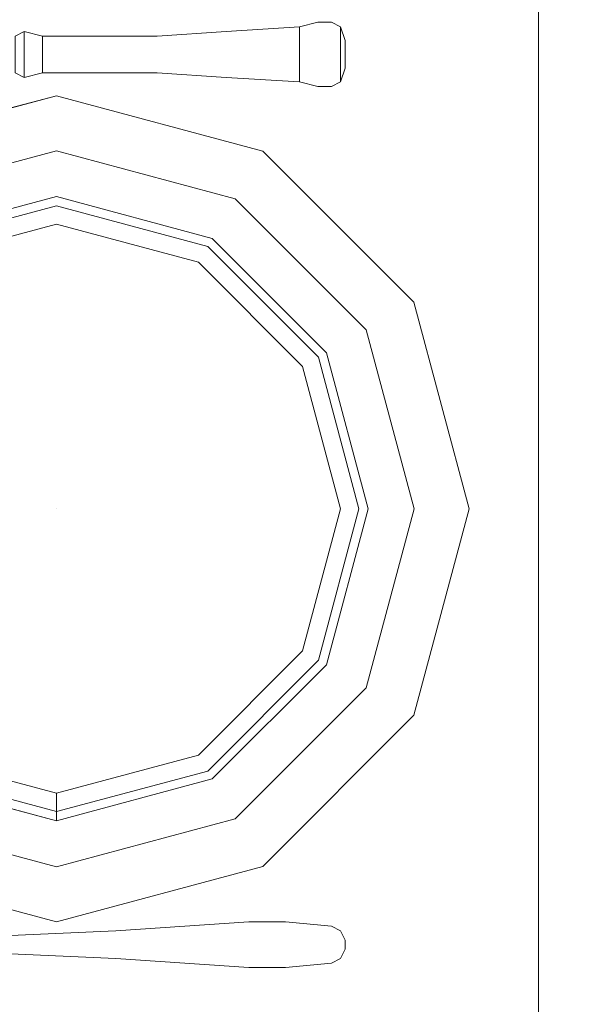
# Model space of a CAD drawing. Units: inches. Extents: x 375 to 1122, y 27 to 1069.
# Tile 36 of 155: x 739.28 to 747.02, y 270.59 to 283.8. Entities that reach past the tile are written whole.
import ezdxf

# ---------------------------------------------------------------- set-up
doc = ezdxf.new("R2010")
doc.units = ezdxf.units.IN
doc.layers.add('A-ANNO-DIMS', color=2, linetype='Continuous', lineweight=18)
doc.layers.add('Furniture', color=30, linetype='Continuous', lineweight=18)
doc.styles.get("Standard").update_dxf_attribs({"font": 'arial.ttf'})
doc.dimstyles.new('ISO-25', dxfattribs={"dimtxt": 12, "dimasz": 2.5, "dimexe": 1.5, "dimexo": 1.5, "dimtad": 1, "dimdec": 1, "dimlunit": 3, "dimtxsty": 'Standard', "dimblk": 'ARCHTICK', "dimcen": 2.5, "dimadec": 0, "dimazin": 0, "dimtfac": 1, "dimtdec": 1, "dimtmove": 0, "dimatfit": 3, "dimfxl": 1.5, "dimfxlon": 1, "dimarcsym": 0})

# ---------------------------------------------------------------- blocks, each defined once
blk = doc.blocks.new('A$C403C54AD')
blk.add_line((0.83575, 1.53256, -0.0006), (1.99923, 1.53256, -0.0006))
at = {"linetype": 'ByBlock'}
for points, invisible_edges in [([(1.72651, 1.50922, -0.02349), (1.72651, 1.49075, -0.02349), (1.66648, 1.47466, -0.02349), (1.65725, 1.49066, -0.02349)], 5), ([(1.72651, 1.47535, -0.03734), (1.72651, 1.50922, -0.02811), (1.65725, 1.49066, -0.02811), (1.67418, 1.46133, -0.03734)], 5), ([(1.79578, 1.49066, -0.02349), (1.78654, 1.47466, -0.02349), (1.72651, 1.49075, -0.02349), (1.72651, 1.50922, -0.02349)], 5), ([(1.77884, 1.46133, -0.03734), (1.79578, 1.49066, -0.02811), (1.72651, 1.50922, -0.02811), (1.72651, 1.47535, -0.03734)], 5), ([(1.65725, 1.49066, -0.02349), (1.66648, 1.47466, -0.02349), (1.62254, 1.43072, -0.02349), (1.60654, 1.43995, -0.02349)], 5), ([(1.67418, 1.46133, -0.03734), (1.65725, 1.49066, -0.02811), (1.60654, 1.43995, -0.02811), (1.63587, 1.42302, -0.03734)], 5), ([(1.72651, 1.49075, -0.02349), (1.72651, 1.47228, -0.02965), (1.67572, 1.45867, -0.02965), (1.66648, 1.47466, -0.02349)], 5), ([(1.78654, 1.47466, -0.02349), (1.7773, 1.45867, -0.02965), (1.72651, 1.47228, -0.02965), (1.72651, 1.49075, -0.02349)], 5), ([(1.81715, 1.42302, -0.03734), (1.84648, 1.43995, -0.02811), (1.79578, 1.49066, -0.02811), (1.77884, 1.46133, -0.03734)], 5), ([(1.84648, 1.43995, -0.02349), (1.83048, 1.43072, -0.02349), (1.78654, 1.47466, -0.02349), (1.79578, 1.49066, -0.02349)], 5), ([(1.66648, 1.47466, -0.02349), (1.67572, 1.45867, -0.02965), (1.63853, 1.42148, -0.02965), (1.62254, 1.43072, -0.02349)], 5), ([(1.72651, 1.46612, -0.04658), (1.72651, 1.47535, -0.03734), (1.67418, 1.46133, -0.03734), (1.6788, 1.45333, -0.04658)], 5), ([(1.77423, 1.45333, -0.04658), (1.77884, 1.46133, -0.03734), (1.72651, 1.47535, -0.03734), (1.72651, 1.46612, -0.04658)], 5), ([(1.83048, 1.43072, -0.02349), (1.81449, 1.42148, -0.02965), (1.7773, 1.45867, -0.02965), (1.78654, 1.47466, -0.02349)], 5), ([(1.72651, 1.47228, -0.02965), (1.72651, 1.37069, -0.02965), (1.72651, 1.37069, -0.02965), (1.67572, 1.45867, -0.02965)], 5), ([(1.7773, 1.45867, -0.02965), (1.72651, 1.37069, -0.02965), (1.72651, 1.37069, -0.02965), (1.72651, 1.47228, -0.02965)], 5), ([(1.6788, 1.45333, -0.04658), (1.67418, 1.46133, -0.03734), (1.63587, 1.42302, -0.03734), (1.64387, 1.4184, -0.04658)], 5), ([(1.80916, 1.4184, -0.04658), (1.81715, 1.42302, -0.03734), (1.77884, 1.46133, -0.03734), (1.77423, 1.45333, -0.04658)], 5), ([(1.67572, 1.45867, -0.02965), (1.72651, 1.37069, -0.02965), (1.72651, 1.37069, -0.02965), (1.63853, 1.42148, -0.02965)], 5), ([(1.81449, 1.42148, -0.02965), (1.72651, 1.37069, -0.02965), (1.72651, 1.37069, -0.02965), (1.7773, 1.45867, -0.02965)], 5), ([(1.60654, 1.43995, -0.02349), (1.62254, 1.43072, -0.02349), (1.60645, 1.37069, -0.02349), (1.58798, 1.37069, -0.02349)], 5), ([(1.63587, 1.42302, -0.03734), (1.60654, 1.43995, -0.02811), (1.58798, 1.37069, -0.02811), (1.62185, 1.37069, -0.03734)], 5), ([(1.83118, 1.37069, -0.03734), (1.86504, 1.37069, -0.02811), (1.84648, 1.43995, -0.02811), (1.81715, 1.42302, -0.03734)], 5), ([(1.86504, 1.37069, -0.02349), (1.84657, 1.37069, -0.02349), (1.83048, 1.43072, -0.02349), (1.84648, 1.43995, -0.02349)], 5), ([(1.62254, 1.43072, -0.02349), (1.63853, 1.42148, -0.02965), (1.62492, 1.37069, -0.02965), (1.60645, 1.37069, -0.02349)], 5), ([(1.84657, 1.37069, -0.02349), (1.8281, 1.37069, -0.02965), (1.81449, 1.42148, -0.02965), (1.83048, 1.43072, -0.02349)], 5), ([(1.64387, 1.4184, -0.04658), (1.63587, 1.42302, -0.03734), (1.62185, 1.37069, -0.03734), (1.63108, 1.37069, -0.04658)], 5), ([(1.63853, 1.42148, -0.02965), (1.72651, 1.37069, -0.02965), (1.72651, 1.37069, -0.02965), (1.62492, 1.37069, -0.02965)], 5), ([(1.8281, 1.37069, -0.02965), (1.72651, 1.37069, -0.02965), (1.72651, 1.37069, -0.02965), (1.81449, 1.42148, -0.02965)], 5), ([(1.82194, 1.37069, -0.04658), (1.83118, 1.37069, -0.03734), (1.81715, 1.42302, -0.03734), (1.80916, 1.4184, -0.04658)], 4), ([(1.58798, 1.37069, -0.02349), (1.60645, 1.37069, -0.02349), (1.62254, 1.31066, -0.02349), (1.60654, 1.30143, -0.02349)], 5), ([(1.62185, 1.37069, -0.03734), (1.58798, 1.37069, -0.02811), (1.60654, 1.30143, -0.02811), (1.63587, 1.31836, -0.03734)], 5), ([(1.60645, 1.37069, -0.02349), (1.62492, 1.37069, -0.02965), (1.63853, 1.3199, -0.02965), (1.62254, 1.31066, -0.02349)], 5), ([(1.63108, 1.37069, -0.04658), (1.62185, 1.37069, -0.03734), (1.63587, 1.31836, -0.03734), (1.64387, 1.32297, -0.04658)], 5), ([(1.62492, 1.37069, -0.02965), (1.72651, 1.37069, -0.02965), (1.72651, 1.37069, -0.02965), (1.63853, 1.3199, -0.02965)], 5), ([(1.63853, 1.3199, -0.02965), (1.72651, 1.37069, -0.02965), (1.72651, 1.37069, -0.02965), (1.67572, 1.28271, -0.02965)], 5), ([(1.67572, 1.28271, -0.02965), (1.72651, 1.37069, -0.02965), (1.72651, 1.37069, -0.02965), (1.72651, 1.2691, -0.02965)], 5), ([(1.72651, 1.2691, -0.02965), (1.72651, 1.37069, -0.02965), (1.72651, 1.37069, -0.02965), (1.7773, 1.28271, -0.02965)], 5), ([(1.81449, 1.3199, -0.02965), (1.72651, 1.37069, -0.02965), (1.72651, 1.37069, -0.02965), (1.8281, 1.37069, -0.02965)], 5), ([(1.7773, 1.28271, -0.02965), (1.72651, 1.37069, -0.02965), (1.72651, 1.37069, -0.02965), (1.81449, 1.3199, -0.02965)], 5), ([(1.83048, 1.31066, -0.02349), (1.81449, 1.3199, -0.02965), (1.8281, 1.37069, -0.02965), (1.84657, 1.37069, -0.02349)], 5), ([(1.81715, 1.31836, -0.03734), (1.84648, 1.30143, -0.02811), (1.86504, 1.37069, -0.02811), (1.83118, 1.37069, -0.03734)], 5), ([(1.84648, 1.30143, -0.02349), (1.83048, 1.31066, -0.02349), (1.84657, 1.37069, -0.02349), (1.86504, 1.37069, -0.02349)], 5)]:
    blk.add_3dface(points, dxfattribs=dict(at, invisible_edges=invisible_edges))
for points in [[(1.72651, 1.50922, -0.02811), (1.72651, 1.50922, -0.02349), (1.65725, 1.49066, -0.02349), (1.65725, 1.49066, -0.02811)], [(1.79578, 1.49066, -0.02811), (1.79578, 1.49066, -0.02349), (1.72651, 1.50922, -0.02349), (1.72651, 1.50922, -0.02811)], [(1.65725, 1.49066, -0.02811), (1.65725, 1.49066, -0.02349), (1.60654, 1.43995, -0.02349), (1.60654, 1.43995, -0.02811)], [(1.84648, 1.43995, -0.02811), (1.84648, 1.43995, -0.02349), (1.79578, 1.49066, -0.02349), (1.79578, 1.49066, -0.02811)], [(1.60654, 1.43995, -0.02811), (1.60654, 1.43995, -0.02349), (1.58798, 1.37069, -0.02349), (1.58798, 1.37069, -0.02811)], [(1.86504, 1.37069, -0.02811), (1.86504, 1.37069, -0.02349), (1.84648, 1.43995, -0.02349), (1.84648, 1.43995, -0.02811)], [(1.58798, 1.37069, -0.02811), (1.58798, 1.37069, -0.02349), (1.60654, 1.30143, -0.02349), (1.60654, 1.30143, -0.02811)], [(1.80916, 1.32297, -0.04658), (1.81715, 1.31836, -0.03734), (1.83118, 1.37069, -0.03734), (1.82194, 1.37069, -0.04658)], [(1.84648, 1.30143, -0.02811), (1.84648, 1.30143, -0.02349), (1.86504, 1.37069, -0.02349), (1.86504, 1.37069, -0.02811)]]:
    blk.add_3dface(points, dxfattribs=at)
for points in [[(1.58337, 1.46612, -0.03734), (1.5649, 1.46612, -0.03734), (1.56951, 1.46766, -0.04042), (1.57875, 1.46766, -0.04042)], [(1.56951, 1.46766, -0.04042), (1.56951, 1.46766, -0.04042), (1.5649, 1.46612, -0.03734), (1.5649, 1.46612, -0.0435)], [(1.58337, 1.46612, -0.0435), (1.5649, 1.46612, -0.0435), (1.56951, 1.46766, -0.04042), (1.57875, 1.46766, -0.04042)], [(1.58337, 1.46612, -0.03734), (1.58337, 1.46612, -0.0435), (1.57875, 1.46766, -0.04042)], [(1.8712, 1.46766, -0.03827), (1.8712, 1.46766, -0.03413), (1.86812, 1.46612, -0.03397), (1.86812, 1.46612, -0.0386)], [(1.87427, 1.46766, -0.03413), (1.87427, 1.46766, -0.03827), (1.8712, 1.46766, -0.03827), (1.8712, 1.46766, -0.03413)], [(1.87735, 1.46612, -0.0386), (1.87735, 1.46612, -0.03397), (1.87427, 1.46766, -0.03413), (1.87427, 1.46766, -0.03827)], [(1.5649, 1.46612, -0.03734), (1.5649, 1.46612, -0.0435), (1.56336, 1.46304, -0.04504), (1.56336, 1.46304, -0.03581)], [(1.56336, 1.46304, -0.03581), (1.56336, 1.46304, -0.04504), (1.56336, 1.45842, -0.04658), (1.56336, 1.45842, -0.03427)], [(1.58491, 1.46304, -0.04504), (1.58491, 1.46304, -0.03581), (1.58337, 1.46612, -0.03734), (1.58337, 1.46612, -0.0435)], [(1.58491, 1.45842, -0.03427), (1.58491, 1.45842, -0.04658), (1.58491, 1.46304, -0.04504), (1.58491, 1.46304, -0.03581)], [(1.86658, 1.46304, -0.03884), (1.86658, 1.46304, -0.03421), (1.86504, 1.44765, -0.03425), (1.86504, 1.44765, -0.03888)], [(1.86812, 1.46612, -0.03397), (1.86812, 1.46612, -0.0386), (1.86658, 1.46304, -0.03884), (1.86658, 1.46304, -0.03421)], [(1.87889, 1.46304, -0.03421), (1.87889, 1.46304, -0.03884), (1.87735, 1.46612, -0.0386), (1.87735, 1.46612, -0.03397)], [(1.88043, 1.44765, -0.03888), (1.88043, 1.44765, -0.03425), (1.87889, 1.46304, -0.03421), (1.87889, 1.46304, -0.03884)], [(1.56336, 1.45842, -0.04658), (1.56336, 1.45842, -0.03427), (1.5649, 1.45227, -0.03581), (1.5649, 1.45227, -0.04504)], [(1.58337, 1.45227, -0.04504), (1.58337, 1.45227, -0.03581), (1.58491, 1.45842, -0.03427), (1.58491, 1.45842, -0.04658)], [(1.5649, 1.45227, -0.03581), (1.5649, 1.45227, -0.04504), (1.56644, 1.42764, -0.04658), (1.56644, 1.42764, -0.03427)], [(1.58183, 1.42764, -0.03427), (1.58183, 1.42764, -0.04658), (1.58337, 1.45227, -0.04504), (1.58337, 1.45227, -0.03581)], [(1.86504, 1.44765, -0.03425), (1.86504, 1.44765, -0.03888), (1.86504, 1.43534, -0.03855), (1.86504, 1.43534, -0.03392)], [(1.88043, 1.43534, -0.03392), (1.88043, 1.43534, -0.03855), (1.88043, 1.44765, -0.03888), (1.88043, 1.44765, -0.03425)], [(1.56644, 1.42764, -0.04658), (1.56644, 1.42764, -0.03427), (1.56797, 1.40455, -0.03427), (1.56797, 1.40455, -0.04658)], [(1.58029, 1.40455, -0.04658), (1.58029, 1.40455, -0.03427), (1.58183, 1.42764, -0.03427), (1.58183, 1.42764, -0.04658)], [(1.56797, 1.40455, -0.03427), (1.56797, 1.40455, -0.04658), (1.56797, 1.36607, -0.04504), (1.56797, 1.36607, -0.03581)], [(1.58029, 1.36607, -0.03581), (1.58029, 1.36607, -0.04504), (1.58029, 1.40455, -0.04658), (1.58029, 1.40455, -0.03427)], [(1.56644, 1.35991, -0.03427), (1.58183, 1.35991, -0.03427), (1.58029, 1.36607, -0.03581), (1.56797, 1.36607, -0.03581)], [(1.56644, 1.35991, -0.04658), (1.58183, 1.35991, -0.04658), (1.58029, 1.36607, -0.04504), (1.56797, 1.36607, -0.04504)], [(1.56797, 1.36607, -0.04504), (1.56797, 1.36607, -0.03581), (1.56644, 1.35991, -0.03427), (1.56644, 1.35991, -0.04658)], [(1.58183, 1.35991, -0.04658), (1.58183, 1.35991, -0.03427), (1.58029, 1.36607, -0.03581), (1.58029, 1.36607, -0.04504)], [(1.58029, 1.35684, -0.03581), (1.56797, 1.35684, -0.03581), (1.56644, 1.35991, -0.03427), (1.58183, 1.35991, -0.03427)], [(1.58029, 1.35684, -0.04504), (1.56797, 1.35684, -0.04504), (1.56644, 1.35991, -0.04658), (1.58183, 1.35991, -0.04658)], [(1.56644, 1.35991, -0.03427), (1.56644, 1.35991, -0.04658), (1.56797, 1.35684, -0.04504), (1.56797, 1.35684, -0.03581)], [(1.58029, 1.35684, -0.03581), (1.58029, 1.35684, -0.04504), (1.58183, 1.35991, -0.04658), (1.58183, 1.35991, -0.03427)]]:
    blk.add_3dface(points)
for points, invisible_edges in [([(1.87427, 1.46766, -0.03413), (1.8712, 1.46766, -0.03413), (1.86812, 1.46612, -0.03397), (1.87735, 1.46612, -0.03397)], 4), ([(1.87427, 1.46766, -0.03827), (1.8712, 1.46766, -0.03827), (1.86812, 1.46612, -0.0386), (1.87735, 1.46612, -0.0386)], 4), ([(1.56336, 1.46304, -0.03581), (1.58491, 1.46304, -0.03581), (1.58337, 1.46612, -0.03734), (1.5649, 1.46612, -0.03734)], 1), ([(1.56336, 1.46304, -0.04504), (1.58491, 1.46304, -0.04504), (1.58337, 1.46612, -0.0435), (1.5649, 1.46612, -0.0435)], 1), ([(1.58491, 1.45842, -0.03427), (1.56336, 1.45842, -0.03427), (1.56336, 1.46304, -0.03581), (1.58491, 1.46304, -0.03581)], 5), ([(1.58491, 1.45842, -0.04658), (1.56336, 1.45842, -0.04658), (1.56336, 1.46304, -0.04504), (1.58491, 1.46304, -0.04504)], 5), ([(1.87889, 1.46304, -0.03421), (1.86658, 1.46304, -0.03421), (1.86504, 1.44765, -0.03425), (1.88043, 1.44765, -0.03425)], 5), ([(1.87889, 1.46304, -0.03884), (1.86658, 1.46304, -0.03884), (1.86504, 1.44765, -0.03888), (1.88043, 1.44765, -0.03888)], 5), ([(1.86812, 1.46612, -0.03397), (1.87735, 1.46612, -0.03397), (1.87889, 1.46304, -0.03421), (1.86658, 1.46304, -0.03421)], 5), ([(1.86812, 1.46612, -0.0386), (1.87735, 1.46612, -0.0386), (1.87889, 1.46304, -0.03884), (1.86658, 1.46304, -0.03884)], 5), ([(1.5649, 1.45227, -0.03581), (1.58337, 1.45227, -0.03581), (1.58491, 1.45842, -0.03427), (1.56336, 1.45842, -0.03427)], 4), ([(1.5649, 1.45227, -0.04504), (1.58337, 1.45227, -0.04504), (1.58491, 1.45842, -0.04658), (1.56336, 1.45842, -0.04658)], 4), ([(1.58183, 1.42764, -0.03427), (1.56644, 1.42764, -0.03427), (1.5649, 1.45227, -0.03581), (1.58337, 1.45227, -0.03581)], 1), ([(1.58183, 1.42764, -0.04658), (1.56644, 1.42764, -0.04658), (1.5649, 1.45227, -0.04504), (1.58337, 1.45227, -0.04504)], 1), ([(1.86504, 1.44765, -0.03425), (1.88043, 1.44765, -0.03425), (1.88043, 1.43534, -0.03392), (1.86504, 1.43534, -0.03392)], 5), ([(1.86504, 1.44765, -0.03888), (1.88043, 1.44765, -0.03888), (1.88043, 1.43534, -0.03855), (1.86504, 1.43534, -0.03855)], 5), ([(1.88043, 1.43534, -0.03392), (1.86504, 1.43534, -0.03392), (1.86812, 1.3907, -0.03153), (1.87735, 1.3907, -0.03153)], 5), ([(1.88043, 1.43534, -0.03855), (1.86504, 1.43534, -0.03855), (1.86812, 1.3907, -0.03461), (1.87735, 1.3907, -0.03461)], 5), ([(1.86504, 1.43534, -0.03855), (1.86504, 1.43534, -0.03392), (1.86812, 1.3907, -0.03153), (1.86812, 1.3907, -0.03461)], 4), ([(1.87735, 1.3907, -0.03461), (1.87735, 1.3907, -0.03153), (1.88043, 1.43534, -0.03392), (1.88043, 1.43534, -0.03855)], 1), ([(1.56797, 1.40455, -0.03427), (1.58029, 1.40455, -0.03427), (1.58183, 1.42764, -0.03427), (1.56644, 1.42764, -0.03427)], 5), ([(1.56797, 1.40455, -0.04658), (1.58029, 1.40455, -0.04658), (1.58183, 1.42764, -0.04658), (1.56644, 1.42764, -0.04658)], 5), ([(1.58029, 1.36607, -0.03581), (1.56797, 1.36607, -0.03581), (1.56797, 1.40455, -0.03427), (1.58029, 1.40455, -0.03427)], 4), ([(1.58029, 1.36607, -0.04504), (1.56797, 1.36607, -0.04504), (1.56797, 1.40455, -0.04658), (1.58029, 1.40455, -0.04658)], 4), ([(1.86812, 1.3907, -0.03153), (1.87735, 1.3907, -0.03153), (1.87581, 1.3553, -0.02863), (1.86966, 1.3553, -0.02863)], 1), ([(1.86812, 1.3907, -0.03153), (1.86812, 1.3907, -0.03461), (1.86966, 1.3553, -0.03122), (1.86966, 1.3553, -0.02863)], 5), ([(1.86812, 1.3907, -0.03461), (1.87735, 1.3907, -0.03461), (1.87581, 1.3553, -0.03122), (1.86966, 1.3553, -0.03122)], 1), ([(1.87581, 1.3553, -0.02863), (1.87581, 1.3553, -0.03122), (1.87735, 1.3907, -0.03461), (1.87735, 1.3907, -0.03153)], 5)]:
    blk.add_3dface(points, dxfattribs=dict(invisible_edges=invisible_edges))
blk = doc.blocks.new('_ArchTick')
at = {"color": 0, "linetype": 'ByBlock', "const_width": 0.15}
blk.add_lwpolyline([(-0.5, -0.5), (0.5, 0.5)], dxfattribs=at)
blk = doc.blocks.new('*D94')
at = {"layer": 'A-ANNO-DIMS', "color": 0, "lineweight": -2, "transparency": 16777216}
for p, q in [((734.007, 117.528), (734.007, 114.528)), ((773.007, 117.528), (773.007, 114.528)), ((734.007, 116.028), (773.007, 116.028))]:
    blk.add_line(p, q, dxfattribs=at)
at = {"layer": 'Defpoints', "color": 0, "transparency": 16777216}
for p in [(734.007, 667.528), (773.007, 667.528), (773.007, 116.028)]:
    blk.add_point(p, dxfattribs=at)
at = {"layer": 'A-ANNO-DIMS', "color": 0, "lineweight": -2, "transparency": 16777216, "xscale": 2.5, "yscale": 2.5, "zscale": 2.5, "rotation": 180}
blk.add_blockref('_ArchTick', (734.007, 116.028), dxfattribs=at)
at = {"layer": 'A-ANNO-DIMS', "color": 0, "lineweight": -2, "transparency": 16777216, "xscale": 2.5, "yscale": 2.5, "zscale": 2.5}
blk.add_blockref('_ArchTick', (773.007, 116.028), dxfattribs=at)
at = {"layer": 'A-ANNO-DIMS', "color": 0, "transparency": 16777216, "insert": (753.507, 122.784), "char_height": 12, "attachment_point": 5}
blk.add_mtext('3\'-3"', dxfattribs=at)

msp = doc.modelspace()

# ---------------------------------------------------------------- block references
at = {"layer": 'Furniture', "xscale": 39.9918517141215, "yscale": 39.9918517141215, "zscale": 39.9918517141215, "rotation": 270}
msp.add_blockref('A$C403C54AD', (684.955, 346.287, 0.024), dxfattribs=at)

# ---------------------------------------------------------------- dimensions: what is measured, and where the dimension line sits
at = {"layer": 'A-ANNO-DIMS'}
dim = msp.add_linear_dim(base=(773.007, 116.028), p1=(734.007, 667.528), p2=(773.007, 667.528), dimstyle='ISO-25', override={"dimdec": 1, "dimlfac": 1, "dimrnd": 0, "dimzin": 1, "dimdsep": 46, "dimlunit": 4, "dimfrac": 2}, dxfattribs=at)
dim.commit()
dim.dimension.update_dxf_attribs({"geometry": '*D94', "text_midpoint": (753.507, 122.784)})

doc.saveas('drawing.dxf')
